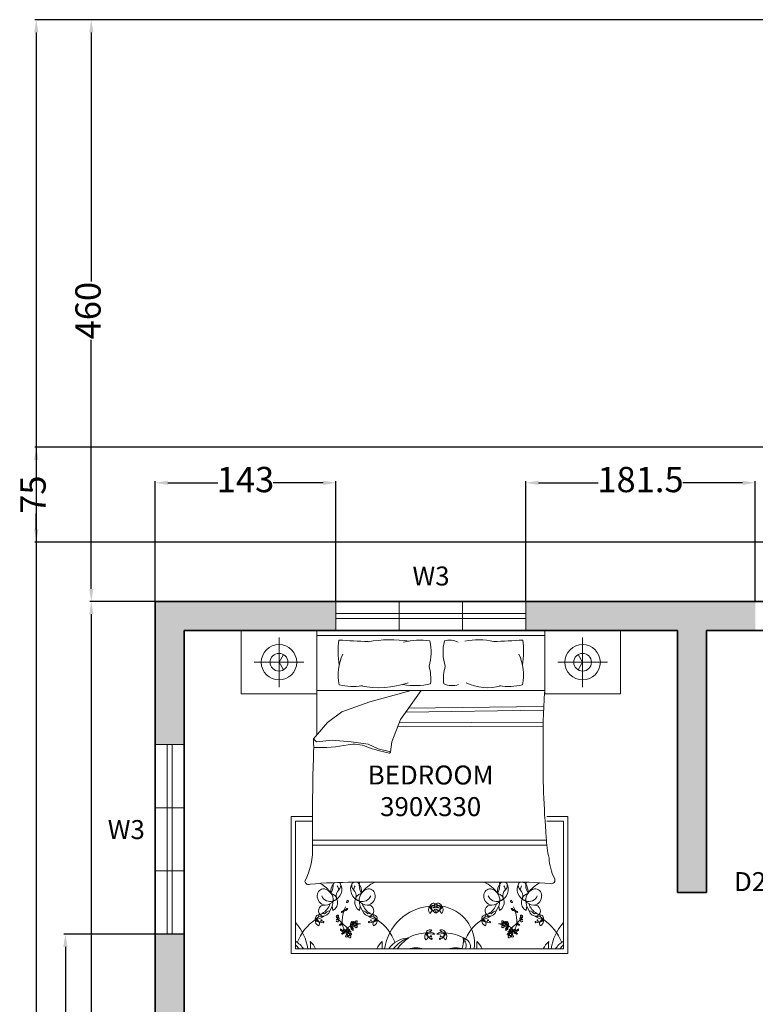
# Model space of a CAD drawing. Units: centimetres. Extents: x 2137 to 3697, y 183 to 2094.
# Tile 7 of 8: x 2163 to 2745, y 1208 to 1987. Entities that reach past the tile are written whole.
import ezdxf

# ---------------------------------------------------------------- set-up
doc = ezdxf.new("R2010")
doc.units = ezdxf.units.CM
for name, color, linetype, lineweight in [('A-ANNO-DIMS', 2, 'Continuous', 18), ('A-ANNO-TEXT', 7, 'Continuous', 18), ('A-AREA-IDEN', 7, 'Continuous', 25), ('A-FURN', 8, 'Continuous', 18), ('A-GLAZ', 4, 'Continuous', 18), ('A-WALL', 7, 'Continuous', 35), ('A-WALL-PATT', 52, 'Continuous', 13)]:
    doc.layers.add(name, color=color, linetype=linetype, lineweight=lineweight)
doc.styles.get("Standard").update_dxf_attribs({"font": 'arial.ttf'})
doc.dimstyles.new('ISO-25', dxfattribs={"dimtxt": 20, "dimasz": 10, "dimexe": 1.25, "dimexo": 0.625, "dimtad": 0, "dimtxsty": 'Standard', "dimcen": 2.5, "dimadec": 0, "dimazin": 0, "dimtfac": 1, "dimtmove": 0, "dimatfit": 3, "dimfxl": 1, "dimarcsym": 0})

# ---------------------------------------------------------------- blocks, each defined once
blk = doc.blocks.new('*D6')
at = {"layer": 'A-ANNO-DIMS', "color": 0, "lineweight": -2, "transparency": 16777216}
for p, q in [((2857.4, 1986.58), (2218.37, 1986.58)), ((2219.62, 1976.58), (2219.62, 1779.67)), ((2219.62, 1536.58), (2219.62, 1733.49)), ((2857.4, 1526.58), (2218.37, 1526.58))]:
    blk.add_line(p, q, dxfattribs=at)
at = {"layer": 'A-ANNO-DIMS', "color": 0, "transparency": 16777216}
for points in [[(2217.95, 1976.58), (2221.28, 1976.58), (2219.62, 1986.58)], [(2217.95, 1536.58), (2221.28, 1536.58), (2219.62, 1526.58)]]:
    blk.add_solid(points, dxfattribs=at)
at = {"layer": 'Defpoints', "color": 0, "transparency": 16777216}
for p in [(2858.02, 1986.58), (2219.62, 1526.58), (2858.02, 1526.58)]:
    blk.add_point(p, dxfattribs=at)
at = {"layer": 'A-ANNO-DIMS', "color": 0, "transparency": 16777216, "insert": (2219.62, 1756.58), "char_height": 20, "attachment_point": 5, "rotation": 90}
blk.add_mtext('460', dxfattribs=at)
blk = doc.blocks.new('*D7')
at = {"layer": 'A-ANNO-DIMS', "color": 0, "lineweight": -2, "transparency": 16777216}
for p, q in [((2269.4, 1526.58), (2218.41, 1526.58)), ((2219.66, 1516.58), (2219.66, 941.09)), ((2219.66, 306.58), (2219.66, 882.07)), ((2269.4, 296.58), (2218.41, 296.58))]:
    blk.add_line(p, q, dxfattribs=at)
at = {"layer": 'A-ANNO-DIMS', "color": 0, "transparency": 16777216}
for points in [[(2217.99, 1516.58), (2221.33, 1516.58), (2219.66, 1526.58)], [(2217.99, 306.58), (2221.33, 306.58), (2219.66, 296.58)]]:
    blk.add_solid(points, dxfattribs=at)
at = {"layer": 'Defpoints', "color": 0, "transparency": 16777216}
for p in [(2270.02, 1526.58), (2219.66, 296.58), (2270.02, 296.58)]:
    blk.add_point(p, dxfattribs=at)
at = {"layer": 'A-ANNO-DIMS', "color": 0, "transparency": 16777216, "insert": (2219.66, 911.58), "char_height": 20, "attachment_point": 5, "rotation": 90}
blk.add_mtext('1230', dxfattribs=at)
blk = doc.blocks.new('BED')
for p, q in [((2442.52, 2474.71), (2742.52, 2474.71)), ((2472.52, 2430.11), (2472.52, 2469.31)), ((2502.52, 2474.71), (2502.52, 2392.37)), ((2682.52, 2470.86), (2502.52, 2470.86)), ((2712.52, 2430.11), (2712.52, 2469.31)), ((2492.12, 2449.71), (2452.92, 2449.71)), ((2692.92, 2449.71), (2732.12, 2449.71)), ((2502.52, 2427.3), (2682.52, 2427.3)), ((2544.19, 2418.38), (2576.9, 2427.3)), ((2584.93, 2427.3), (2568.49, 2404.42)), ((2522.31, 2410.49), (2544.19, 2418.38)), ((2681.71, 2414.84), (2574.9, 2413.34)), ((2510.77, 2401.99), (2522.31, 2410.49)), ((2681.6, 2411.76), (2572.66, 2410.22)), ((2499.83, 2389.24), (2510.77, 2401.99)), ((2568.49, 2404.42), (2561.81, 2386.81)), ((2681.46, 2399.23), (2566.35, 2398.76)), ((2681.44, 2402.31), (2567.52, 2401.86)), ((2502.26, 2386.81), (2499.83, 2389.24)), ((2514.41, 2388.02), (2502.26, 2386.81)), ((2529.61, 2386.81), (2514.41, 2388.02)), ((2542.97, 2384.99), (2529.61, 2386.81)), ((2550.87, 2381.34), (2542.97, 2384.99)), ((2561.81, 2386.81), (2560.59, 2378.91)), ((2560.59, 2378.91), (2550.87, 2381.34)), ((2482.11, 2327.65), (2499.08, 2327.65)), ((2482.11, 2219.58), (2482.11, 2327.65)), ((2684.19, 2327.65), (2700.83, 2327.65)), ((2700.83, 2327.65), (2700.83, 2219.58)), ((2499.08, 2324.17), (2485.59, 2324.17)), ((2485.59, 2324.17), (2485.59, 2223.06)), ((2697.35, 2324.17), (2684.13, 2324.17)), ((2697.35, 2223.06), (2697.35, 2324.17)), ((2683.88, 2308.94), (2499.06, 2308.94)), ((2684.17, 2305.2), (2499.06, 2305.2)), ((2653.42, 2275.73), (2531.62, 2275.73)), ((2515.15, 2253.47), (2514.49, 2256.86)), ((2536.12, 2253.47), (2536.78, 2256.86)), ((2646.82, 2253.47), (2646.16, 2256.86)), ((2667.79, 2253.47), (2668.45, 2256.86)), ((2700.83, 2219.58), (2482.11, 2219.58)), ((2485.59, 2223.06), (2697.35, 2223.06))]:
    blk.add_line(p, q)
for points in [[(2502.52, 2424.71), (2442.52, 2424.71), (2442.52, 2474.71)], [(2682.52, 2474.71), (2682.52, 2424.71), (2742.52, 2424.71), (2742.52, 2474.71)], [(2472.52, 2449.71), (2476.02, 2455.77)], [(2712.52, 2449.71), (2709.02, 2455.77)], [(2472.52, 2449.71), (2476.02, 2443.65)], [(2712.52, 2449.71), (2709.02, 2443.65)]]:
    blk.add_lwpolyline(points)
for points in [[(2519.75, 2467.23, 0.074897), (2520.11, 2447.64, -0.472817)], [(2591.11, 2446.54, 0.14099), (2591.71, 2466.53, 0.235245)], [(2603.92, 2446.54, -0.14099), (2603.32, 2466.53, -0.235245)], [(2665.29, 2467.23, -0.074897), (2664.92, 2447.64, 0.472817)], [(2499.2, 2361.77, 0.001242), (2499.06, 2304.85, -0.127202), (2493.05, 2276.48)], [(2683.8, 2311.3, 0.056112), (2685.97, 2294.79, 0.095341), (2690.19, 2278.9)]]:
    blk.add_lwpolyline(points, format="xyb")
for centre, radius in [((2472.52, 2449.71), 14), ((2712.52, 2449.71), 14), ((2472.52, 2449.71), 7), ((2712.52, 2449.71), 7), ((2532.49, 2242.6), 0.764), ((2650.46, 2242.6), 0.764), ((2527.49, 2234.55), 0.764), ((2655.45, 2234.55), 0.764)]:
    blk.add_circle(centre, radius)
for centre, radius, start, end in [((2685.11, 5322.24), 2859.79, 266.68521, 267.14978), ((2560.85, 2358.67), 108.8, 82.21958, 99.49698), ((2583.83, 2413.66), 53.46, 81.52493, 103.95996), ((2607.44, 2452.27), 14.84, 63.34374, 106.10256), ((2629.68, 2414.74), 52.74, 76.34271, 101.1841), ((2499.93, 5322.24), 2859.79, 272.85022, 273.31479), ((2557.97, 2439.77), 38.67, 155.1316, 191.75834), ((2627.07, 2439.77), 38.67, 348.24166, 24.8684), ((2555.75, 2436.51), 36.76, 354.01289, 15.82928), ((2639.29, 2436.51), 36.76, 164.17072, 185.98711), ((2530.45, 2470.74), 40.2, 255.10393, 281.03689), ((2551.61, 2499.32), 69.73, 258.03974, 289.26152), ((2579.84, 2484.1), 52.9, 259.86169, 283.62376), ((2609.45, 2447.1), 15.9, 245.01826, 288.54073), ((2637.23, 2467.78), 38.19, 243.87611, 286.17464), ((2654.58, 2470.74), 40.2, 258.96311, 284.89607), ((3220.32, 2390.64), 539.05, 176.09997, 180.92818), ((2224.76, 2381.78), 275.17, 355.82941, 1.55305), ((2504.97, 2495.47), 113.22, 267.45188, 281.3392), ((2532.03, 2360.52), 24.42, 66.26158, 101.3392), ((2581.42, 2492.28), 116.34, 250.11942, 259.33829), ((2559.91, 2378.67), 0.724, 268.86235, 19.75363), ((3384.42, 2371.04), 703.17, 179.11454, 184.87351), ((2495.81, 2276.67), 2.77, 183.97998, 297.34124), ((2528.04, 1963.45), 312.3, 89.34325, 95.68869), ((2494.64, 2254.6), 22.71, 33.66712, 63.29966), ((2525.07, 2268.11), 11.57, 145.78505, 184.73037), ((2502.97, 2273.51), 12.43, 328.82178, 9.15542), ((2518.36, 2272.41), 3.61, 120.0293, 142.32497), ((2512.59, 2270.28), 9.56, 289.28218, 29.1751), ((2516.83, 2273.13), 4.49, 311.56531, 23.83541), ((2518.36, 2272.41), 3.61, 44.45169, 63.55801), ((2538.68, 2270.28), 9.56, 150.8249, 250.71782), ((2534.44, 2273.13), 4.49, 156.16459, 228.43469), ((2532.91, 2272.41), 3.61, 113.22901, 135.54831), ((2532.91, 2272.41), 3.61, 37.67503, 66.71436), ((2526.21, 2268.11), 11.57, 355.26963, 34.21495), ((2548.31, 2273.51), 12.43, 169.71335, 211.17822), ((2556.64, 2254.6), 22.71, 111.49413, 146.33288), ((2626.3, 2254.6), 22.71, 33.66712, 68.50587), ((2656.73, 2268.11), 11.57, 145.78505, 184.73037), ((2634.63, 2273.51), 12.43, 328.82178, 10.28665), ((2650.03, 2272.41), 3.61, 113.28564, 142.32497), ((2644.26, 2270.28), 9.56, 289.28218, 29.1751), ((2650.03, 2272.41), 3.61, 44.45169, 66.71436), ((2648.5, 2273.13), 4.49, 311.56531, 23.83541), ((2662.61, 1983.95), 291.92, 85.24024, 91.80351), ((2670.35, 2270.28), 9.56, 150.8249, 250.71782), ((2666.11, 2273.13), 4.49, 156.16459, 228.43469), ((2664.58, 2272.41), 3.61, 106.63434, 135.54831), ((2664.58, 2272.41), 3.61, 37.67503, 72.58143), ((2657.87, 2268.11), 11.57, 355.26963, 34.21495), ((2679.98, 2273.51), 12.43, 169.24899, 211.17822), ((2688.3, 2254.6), 22.71, 113.64533, 146.33288), ((2687.92, 2277.37), 2.73, 246.52186, 33.82642), ((2509.94, 2264.78), 7.17, 174.94485, 262.88575), ((2507.86, 2265.5), 5.07, 84.48557, 181.05378), ((2506.31, 2261.76), 9.02, 355.29334, 76.921), ((2511.44, 2259.94), 7.46, 299.90854, 73.1337), ((2523.89, 2265.16), 6.15, 131.56531, 195.14713), ((2511.15, 2268.55), 8.62, 7.43599, 29.91487), ((2527.38, 2265.16), 6.15, 344.85287, 48.43469), ((2540.13, 2268.55), 8.62, 150.08513, 172.56401), ((2539.84, 2259.94), 7.46, 106.8663, 240.09146), ((2544.97, 2261.76), 9.02, 103.079, 184.70666), ((2541.33, 2264.78), 7.17, 277.11425, 5.05515), ((2543.41, 2265.5), 5.07, 358.94622, 95.51443), ((2641.61, 2264.78), 7.17, 174.94485, 262.88575), ((2639.53, 2265.5), 5.07, 84.48557, 181.05378), ((2637.98, 2261.76), 9.02, 355.29334, 76.921), ((2643.1, 2259.94), 7.46, 299.90854, 73.1337), ((2655.56, 2265.16), 6.15, 131.56531, 195.14713), ((2642.81, 2268.55), 8.62, 7.43599, 29.91487), ((2659.05, 2265.16), 6.15, 344.85287, 48.43469), ((2671.79, 2268.55), 8.62, 150.08513, 172.56401), ((2671.51, 2259.94), 7.46, 106.8663, 240.09146), ((2676.63, 2261.76), 9.02, 103.079, 184.70666), ((2673, 2264.78), 7.17, 277.11425, 5.05515), ((2675.08, 2265.5), 5.07, 358.94622, 95.51443), ((2508.29, 2253.23), 4.5, 80.26398, 250.86884), ((2512.76, 2267.5), 6.96, 201.58187, 291.42215), ((2499.37, 2263.14), 14.16, 301.26137, 341.7045), ((2508.7, 2266.37), 8.71, 272.3591, 324.04014), ((2499.23, 2262), 16.1, 326.28828, 356.5076), ((2525.07, 2268.11), 11.57, 212.70113, 216.34448), ((2516.16, 2263.07), 1.86, 257.30406, 15.14713), ((2526.5, 2260.25), 0.578, 102.70507, 280.43845), ((2526.43, 2260.6), 0.94, 280.43845, 100.41356), ((2535.12, 2263.07), 1.86, 164.85287, 282.69594), ((2526.21, 2268.11), 11.57, 323.65552, 327.29887), ((2542.58, 2266.37), 8.71, 215.95986, 267.6409), ((2538.52, 2267.5), 6.96, 248.57785, 338.41813), ((2552.04, 2262), 16.1, 183.4924, 213.71172), ((2551.91, 2263.14), 14.16, 198.2955, 238.73863), ((2542.98, 2253.23), 4.5, 289.13116, 99.73602), ((2594.92, 2255.93), 3.25, 63.02737, 163.80375), ((2591.63, 2263.52), 6.69, 271.45846, 315.37266), ((2598.02, 2255.93), 3.25, 16.19625, 116.97263), ((2601.31, 2263.52), 6.69, 224.62734, 268.54154), ((2639.96, 2253.23), 4.5, 80.26398, 250.86884), ((2644.43, 2267.5), 6.96, 201.58187, 291.42215), ((2631.03, 2263.14), 14.16, 301.26137, 341.7045), ((2640.36, 2266.37), 8.71, 272.3591, 324.04014), ((2630.9, 2262), 16.1, 326.28828, 356.5076), ((2656.73, 2268.11), 11.57, 212.70113, 216.34448), ((2647.82, 2263.07), 1.86, 257.30406, 15.14713), ((2656.51, 2260.6), 0.94, 79.58644, 259.56155), ((2656.44, 2260.25), 0.578, 259.56155, 77.29493), ((2666.78, 2263.07), 1.86, 164.85287, 282.69594), ((2657.87, 2268.11), 11.57, 323.65552, 327.29887), ((2674.25, 2266.37), 8.71, 215.95986, 267.6409), ((2670.18, 2267.5), 6.96, 248.57785, 338.41813), ((2683.71, 2262), 16.1, 183.4924, 213.71172), ((2683.58, 2263.14), 14.16, 198.2955, 238.73863), ((2674.65, 2253.23), 4.5, 289.13116, 99.73602), ((2504.48, 2247), 3.25, 92.95159, 193.72796), ((2497.84, 2251.95), 6.69, 301.38267, 345.29688), ((2507.37, 2248.35), 2.76, 63.97555, 143.26805), ((2507.21, 2254.58), 5.62, 265.96902, 344.3045), ((2513.27, 2247.11), 5.99, 96.1662, 141.58255), ((2518.96, 2249.23), 0.59, 345.23556, 144.9248), ((2523.19, 2251.31), 1.58, 101.32561, 154.46214), ((2520.92, 2256.65), 4.74, 280.25878, 300.65599), ((2522.01, 2260.45), 8.46, 268.32639, 277.13024), ((2547.29, 2245.15), 24.85, 163.58418, 183.82768), ((2519.89, 2256.64), 4.82, 308.21012, 316.30712), ((2522.85, 2253.47), 1.44, 278.34322, 4.28685), ((2522.06, 2254.74), 2.51, 300.65599, 332.63414), ((2523.94, 2253.08), 0.611, 55.76575, 157.44165), ((2547.29, 2245.15), 24.85, 153.0032, 159.89408), ((2524.9, 2253.65), 0.611, 84.37838, 186.05427), ((2524.32, 2256.1), 2.51, 269.18588, 301.16403), ((2525.06, 2254.8), 1.44, 237.53317, 323.47681), ((2523.67, 2258.9), 4.82, 285.51291, 293.60991), ((2526.81, 2253.48), 1.58, 87.35788, 140.49441), ((2523.17, 2258), 4.74, 301.16403, 321.56124), ((2519.31, 2258.83), 8.46, 324.68979, 333.49364), ((2538.01, 2247.11), 5.99, 38.41745, 83.8338), ((2544.06, 2254.58), 5.62, 195.6955, 274.03098), ((2543.91, 2248.35), 2.76, 36.73195, 116.02445), ((2546.8, 2247), 3.25, 346.27204, 87.04841), ((2553.44, 2251.95), 6.69, 194.70312, 238.61733), ((2594.85, 2217.78), 39.18, 94.46233, 172.25504), ((2595.02, 2253.92), 4.34, 137.78732, 219.11446), ((2590.09, 2254.05), 3.27, 298.5391, 58.36268), ((2594.35, 2251.19), 6.19, 45.54113, 114.31008), ((2600, 2282.98), 27.41, 252.59304, 267.25817), ((2595, 2256.71), 3.2, 177.75849, 283.85198), ((2601.17, 2260.05), 9.91, 198.91595, 238.01098), ((2598.59, 2251.19), 6.19, 65.68992, 134.45887), ((2592.94, 2282.98), 27.41, 272.74183, 287.40696), ((2595.67, 2254.01), 0.424, 283.85198, 219.92454), ((2596.18, 2252.06), 0.487, 238.01098, 71.55918), ((2596.26, 2252.29), 0.236, 71.55918, 188.01668), ((2596.76, 2252.06), 0.487, 108.44082, 301.98902), ((2596.68, 2252.29), 0.236, 351.98332, 108.44082), ((2597.23, 2254.17), 0.255, 320.19092, 256.02088), ((2591.77, 2260.05), 9.91, 301.98902, 341.08405), ((2597.94, 2256.71), 3.2, 256.14802, 2.24151), ((2602.86, 2254.05), 3.27, 121.63732, 241.4609), ((2597.92, 2253.92), 4.34, 320.88554, 42.21268), ((2596.83, 2226.82), 30.32, 352.86355, 81.81966), ((2636.14, 2247), 3.25, 92.95159, 193.72796), ((2629.51, 2251.95), 6.69, 301.38267, 345.29688), ((2639.03, 2248.35), 2.76, 63.97555, 143.26805), ((2638.88, 2254.58), 5.62, 265.96902, 344.3045), ((2644.93, 2247.11), 5.99, 96.1662, 141.58255), ((2656.13, 2253.48), 1.58, 39.50559, 92.64212), ((2659.77, 2258), 4.74, 218.43876, 238.83597), ((2663.63, 2258.83), 8.46, 206.50636, 215.31021), ((2657.88, 2254.8), 1.44, 216.52319, 302.46683), ((2658.62, 2256.1), 2.51, 238.83597, 270.81412), ((2659.27, 2258.9), 4.82, 246.39009, 254.48709), ((2635.65, 2245.15), 24.85, 20.10592, 26.9968), ((2658.05, 2253.65), 0.611, 353.94573, 95.62162), ((2659, 2253.08), 0.611, 22.55835, 124.23425), ((2660.09, 2253.47), 1.44, 175.71315, 261.65678), ((2660.89, 2254.74), 2.51, 207.36586, 239.34401), ((2635.65, 2245.15), 24.85, 356.17232, 16.41582), ((2663.05, 2256.64), 4.82, 223.69288, 231.78988), ((2662.02, 2256.65), 4.74, 239.34401, 259.74122), ((2660.93, 2260.45), 8.46, 262.86976, 271.67361), ((2659.76, 2251.31), 1.58, 25.53786, 78.67439), ((2663.98, 2249.23), 0.59, 35.0752, 194.76444), ((2675.73, 2254.58), 5.62, 195.6955, 274.03098), ((2669.67, 2247.11), 5.99, 38.41745, 83.8338), ((2675.58, 2248.35), 2.76, 36.73195, 116.02445), ((2685.1, 2251.95), 6.69, 194.70312, 238.61733), ((2678.46, 2247), 3.25, 346.27204, 87.04841), ((2456.43, 2217.78), 39.18, 7.74496, 41.8856), ((2523.45, 2213.9), 39.18, 124.38655, 158.59079), ((2505.57, 2245.31), 4.34, 167.71153, 249.03868), ((2506.35, 2242.61), 6.19, 75.46535, 144.23429), ((2495.38, 2272.99), 27.41, 282.51726, 297.18239), ((2501.23, 2242.96), 3.27, 328.46331, 88.28689), ((2507.84, 2253.69), 9.91, 228.84017, 267.9352), ((2504.16, 2247.72), 3.2, 207.6827, 313.77619), ((2506.09, 2245.71), 0.424, 313.77619, 249.71835), ((2507.46, 2244.52), 0.236, 101.4834, 217.94089), ((2507.5, 2244.28), 0.487, 267.9352, 101.4834), ((2518.73, 2248.32), 1.27, 101.56373, 142.6358), ((2517.68, 2247.14), 0.764, 273.27684, 86.72316), ((2518.72, 2245.73), 1.26, 217.76209, 259.04026), ((2518.57, 2247.86), 0.73, 91.10805, 181.86747), ((2520.08, 2247.41), 2.32, 203.42757, 227.61037), ((2519.34, 2246.4), 1.58, 80.3487, 133.65382), ((2519.06, 2247.7), 1.25, 229.78892, 317.67915), ((2517.71, 2249.32), 1.84, 288.72627, 352.50315), ((2517.65, 2245.06), 1.78, 355.05304, 68.36176), ((2519.04, 2244.75), 2.5, 83.08516, 105.71709), ((2518.83, 2244.95), 0.586, 232.47371, 355.05304), ((2501.72, 2224.01), 28.48, 43.15413, 52.0459), ((2519.5, 2247.3), 0.658, 317.67915, 80.3487), ((2521.4, 2241.21), 1.58, 101.32561, 154.46214), ((2519.13, 2246.56), 4.74, 280.25878, 300.65599), ((2520.22, 2250.35), 8.46, 268.32639, 277.13024), ((2518.11, 2246.55), 4.82, 308.21012, 316.30712), ((2521.07, 2243.38), 1.44, 278.34322, 4.28685), ((2520.27, 2244.64), 2.51, 300.65599, 332.63414), ((2522.16, 2242.98), 0.611, 55.76575, 157.44165), ((2534.91, 2244.52), 12.46, 184.75602, 209.20408), ((2552.85, 2271.04), 40.99, 222.24124, 232.17444), ((2528.5, 2242.96), 2.12, 272.84988, 356.12261), ((2526.64, 2243.74), 3.48, 304.53686, 16.36991), ((2527, 2242.14), 2.05, 321.76073, 7.92519), ((2531.47, 2242.76), 2.46, 127.31045, 187.92519), ((2528.09, 2243.04), 2.53, 355.01064, 41.65801), ((2532.28, 2240.29), 2.41, 104.75581, 148.0499), ((2531.64, 2243.66), 1.04, 126.10456, 271.42811), ((2531.53, 2243.95), 0.749, 353.75256, 131.70535), ((2531.35, 2241.96), 0.506, 262.90601, 7.13198), ((2530.82, 2243.06), 1.05, 0.06451, 61.15075), ((2531.07, 2243.95), 1.2, 311.84125, 355.78771), ((2533.54, 2243.78), 1.27, 101.56373, 176.36503), ((2533.38, 2243.32), 0.73, 91.10805, 181.86747), ((2534.89, 2242.87), 2.32, 203.42757, 227.61037), ((2534.15, 2241.86), 1.58, 80.3487, 133.65382), ((2533.87, 2243.16), 1.25, 229.78892, 317.67915), ((2532.52, 2244.78), 1.84, 288.72627, 352.50315), ((2532.46, 2240.51), 1.78, 355.05304, 68.36176), ((2533.85, 2240.21), 2.5, 83.08516, 105.71709), ((2533.77, 2244.69), 0.59, 345.23556, 144.9248), ((2534.31, 2242.76), 0.658, 317.67915, 80.3487), ((2536.2, 2227.98), 14.94, 87.10709, 94.75853), ((2543.77, 2244.28), 0.487, 78.5166, 272.0648), ((2544.93, 2242.61), 6.19, 35.76571, 104.53465), ((2555.89, 2272.99), 27.41, 242.81761, 257.48274), ((2543.43, 2253.69), 9.91, 272.0648, 311.15983), ((2543.82, 2244.52), 0.236, 322.05911, 78.5166), ((2547.11, 2247.72), 3.2, 226.22381, 332.3173), ((2545.24, 2245.88), 0.255, 290.26671, 226.22708), ((2550.05, 2242.96), 3.27, 91.71311, 211.53669), ((2545.71, 2245.31), 4.34, 290.96132, 12.28847), ((2527.83, 2213.9), 39.18, 21.40921, 55.61345), ((2655.12, 2213.9), 39.18, 124.38655, 158.59079), ((2637.23, 2245.31), 4.34, 167.71153, 249.03868), ((2638.02, 2242.61), 6.19, 75.46535, 144.23429), ((2627.05, 2272.99), 27.41, 282.51726, 297.18239), ((2635.83, 2247.72), 3.2, 207.6827, 313.77619), ((2639.51, 2253.69), 9.91, 228.84017, 267.9352), ((2632.89, 2242.96), 3.27, 328.46331, 88.28689), ((2637.75, 2245.71), 0.424, 313.77619, 249.71835), ((2639.12, 2244.52), 0.236, 101.4834, 217.94089), ((2639.17, 2244.28), 0.487, 267.9352, 101.4834), ((2646.75, 2227.98), 14.94, 85.24147, 92.89291), ((2648.64, 2242.76), 0.658, 99.6513, 222.32085), ((2649.07, 2243.16), 1.25, 222.32085, 310.21108), ((2648.79, 2241.86), 1.58, 46.34618, 99.6513), ((2649.17, 2244.69), 0.59, 35.0752, 194.76444), ((2650.42, 2244.78), 1.84, 187.49685, 251.27373), ((2650.48, 2240.51), 1.78, 111.63824, 184.94696), ((2649.09, 2240.21), 2.5, 74.28291, 96.91484), ((2649.56, 2243.32), 0.73, 358.13253, 88.89195), ((2648.05, 2242.87), 2.32, 312.38963, 336.57243), ((2649.4, 2243.78), 1.27, 3.63497, 78.43627), ((2651.41, 2243.95), 0.749, 48.29465, 186.24744), ((2651.87, 2243.95), 1.2, 184.21229, 228.15875), ((2652.12, 2243.06), 1.05, 118.84925, 179.93549), ((2651.59, 2241.96), 0.506, 172.86802, 277.09399), ((2651.3, 2243.66), 1.04, 268.57189, 53.89544), ((2650.66, 2240.29), 2.41, 31.9501, 75.24419), ((2654.85, 2243.04), 2.53, 138.34199, 184.98936), ((2654.44, 2242.96), 2.12, 183.87739, 267.15012), ((2656.3, 2243.74), 3.48, 163.63009, 235.46314), ((2651.47, 2242.76), 2.46, 352.07481, 52.68955), ((2655.94, 2242.14), 2.05, 172.07481, 218.23927), ((2630.09, 2271.04), 40.99, 307.82556, 317.75876), ((2648.03, 2244.52), 12.46, 330.79592, 355.24398), ((2681.22, 2224.01), 28.48, 127.9541, 136.84587), ((2660.78, 2242.98), 0.611, 22.55835, 124.23425), ((2661.88, 2243.38), 1.44, 175.71315, 261.65678), ((2662.67, 2244.64), 2.51, 207.36586, 239.34401), ((2664.83, 2246.55), 4.82, 223.69288, 231.78988), ((2663.81, 2246.56), 4.74, 239.34401, 259.74122), ((2662.72, 2250.35), 8.46, 262.86976, 271.67361), ((2661.54, 2241.21), 1.58, 25.53786, 78.67439), ((2663.45, 2247.3), 0.658, 99.6513, 222.32085), ((2663.88, 2247.7), 1.25, 222.32085, 310.21108), ((2663.6, 2246.4), 1.58, 46.34618, 99.6513), ((2665.23, 2249.32), 1.84, 187.49685, 251.27373), ((2665.29, 2245.06), 1.78, 111.63824, 184.94696), ((2664.11, 2244.95), 0.586, 184.94696, 307.52629), ((2663.9, 2244.75), 2.5, 74.28291, 96.91484), ((2664.38, 2247.86), 0.73, 358.13253, 88.89195), ((2662.86, 2247.41), 2.32, 312.38963, 336.57243), ((2664.21, 2248.32), 1.27, 37.3642, 78.43627), ((2664.23, 2245.73), 1.26, 280.95974, 322.23791), ((2665.27, 2247.14), 0.764, 93.27684, 266.72316), ((2675.44, 2244.28), 0.487, 78.5166, 272.0648), ((2676.59, 2242.61), 6.19, 35.76571, 104.53465), ((2687.56, 2272.99), 27.41, 242.81761, 257.48274), ((2675.1, 2253.69), 9.91, 272.0648, 311.15983), ((2675.49, 2244.52), 0.236, 322.05911, 78.5166), ((2678.78, 2247.72), 3.2, 226.22381, 332.3173), ((2676.9, 2245.88), 0.255, 290.26671, 226.22708), ((2681.72, 2242.96), 3.27, 91.71311, 211.53669), ((2677.37, 2245.31), 4.34, 290.96132, 12.28847), ((2659.49, 2213.9), 39.18, 21.40921, 55.61345), ((2726.52, 2217.78), 39.18, 138.1144, 172.25504), ((2521.93, 2238.45), 0.853, 146.86359, 236.90213), ((2533.96, 2257.24), 22.32, 235.1882, 238.88441), ((2523.39, 2239.69), 2.31, 199.47987, 267.68284), ((2523.14, 2238.82), 1.99, 212.81548, 277.39917), ((2521.98, 2237.49), 2.31, 266.97007, 338.29129), ((2509.81, 2253.97), 22.32, 302.6784, 306.37461), ((2522.56, 2235.66), 0.853, 214.3538, 304.39233), ((2522.88, 2238.89), 0.883, 238.88441, 314.26458), ((2522.69, 2236.91), 1.99, 280.30568, 17.1958), ((2522.52, 2236.71), 0.883, 306.37461, 21.75478), ((2523.96, 2237.28), 0.666, 19.36054, 201.75478), ((2523.96, 2237.78), 0.666, 311.87034, 134.26458), ((2536.49, 2231.71), 13.31, 153.78194, 158.29129), ((2525.9, 2240.8), 3.48, 247.23048, 319.06353), ((2524.75, 2239.63), 2.05, 264.45436, 310.61881), ((2534.91, 2244.52), 12.46, 214.00334, 222.49171), ((2526.25, 2238.81), 2.12, 218.32082, 298.81623), ((2536.2, 2227.98), 14.94, 120.54402, 139.81798), ((2527.28, 2232.24), 2.41, 104.75581, 148.0499), ((2526.65, 2235.61), 1.04, 126.10456, 271.42811), ((2526.53, 2235.89), 0.749, 353.75256, 131.70535), ((2527.69, 2236.2), 2.46, 70.00407, 130.61881), ((2525.83, 2235), 1.05, 0.06451, 61.15075), ((2526.08, 2235.9), 1.2, 311.84125, 355.78771), ((2526.09, 2239.2), 2.53, 297.70426, 344.35163), ((2528.55, 2235.73), 1.27, 101.56373, 176.36503), ((2528.38, 2235.27), 0.73, 91.10805, 181.86747), ((2529.15, 2233.8), 1.58, 80.3487, 133.65382), ((2528.87, 2235.11), 1.25, 229.78892, 317.67915), ((2527.52, 2236.73), 1.84, 288.72627, 352.50315), ((2527.46, 2232.46), 1.78, 355.05304, 68.36176), ((2528.85, 2232.16), 2.5, 83.08516, 105.71709), ((2528.77, 2236.64), 0.59, 345.23556, 144.9248), ((2527.43, 2239.19), 2.05, 8.72271, 54.88717), ((2527.54, 2237.55), 3.48, 0.278, 72.11105), ((2529.1, 2238.83), 2.12, 20.5253, 88.5375), ((2529.31, 2234.71), 0.658, 317.67915, 80.3487), ((2531.89, 2239.88), 2.46, 188.72271, 249.33746), ((2530.88, 2241.17), 0.757, 148.0499, 225.62681), ((2536.2, 2227.98), 14.94, 113.05007, 113.84774), ((2530.93, 2242.02), 1.51, 247.40857, 351.43859), ((2528.73, 2238.64), 2.53, 334.9899, 21.63727), ((2533.53, 2241.19), 1.26, 151.21959, 259.04026), ((2533.64, 2240.41), 0.586, 232.47371, 355.05304), ((2591.85, 2196.79), 39.18, 94.46233, 117.4146), ((2592.02, 2232.93), 4.34, 137.78732, 219.11446), ((2587.09, 2233.07), 3.27, 298.5391, 58.36268), ((2591.92, 2234.94), 3.25, 63.02737, 163.80375), ((2588.63, 2242.54), 6.69, 271.45846, 315.37266), ((2591.35, 2230.21), 6.19, 45.54113, 114.31008), ((2598.17, 2239.06), 9.91, 198.91595, 238.01098), ((2597, 2262), 27.41, 252.59304, 267.25817), ((2592, 2235.73), 3.2, 177.75849, 283.85198), ((2601.59, 2230.21), 6.19, 65.68992, 134.45887), ((2595.94, 2262), 27.41, 272.74183, 287.40696), ((2601.02, 2234.94), 3.25, 16.19625, 116.97263), ((2604.31, 2242.54), 6.69, 224.62734, 268.54154), ((2594.77, 2239.06), 9.91, 301.98902, 341.08405), ((2600.94, 2235.73), 3.2, 256.14802, 2.24151), ((2605.86, 2233.07), 3.27, 121.63732, 241.4609), ((2600.92, 2232.93), 4.34, 320.88554, 42.21268), ((2601.09, 2196.79), 39.18, 62.5854, 85.53767), ((2649.3, 2240.41), 0.586, 184.94696, 307.52629), ((2649.41, 2241.19), 1.26, 280.95974, 28.78041), ((2652.01, 2242.02), 1.51, 188.56141, 292.59143), ((2654.21, 2238.64), 2.53, 158.36273, 205.0101), ((2653.84, 2238.83), 2.12, 91.4625, 159.4747), ((2655.4, 2237.55), 3.48, 107.88895, 179.722), ((2651.05, 2239.88), 2.46, 290.66254, 351.27729), ((2652.06, 2241.17), 0.757, 314.37319, 31.9501), ((2646.75, 2227.98), 14.94, 66.15226, 66.94993), ((2653.63, 2234.71), 0.658, 99.6513, 222.32085), ((2654.07, 2235.11), 1.25, 222.32085, 310.21108), ((2655.51, 2239.19), 2.05, 125.11283, 171.27729), ((2653.79, 2233.8), 1.58, 46.34618, 99.6513), ((2654.17, 2236.64), 0.59, 35.0752, 194.76444), ((2655.42, 2236.73), 1.84, 187.49685, 251.27373), ((2655.48, 2232.46), 1.78, 111.63824, 184.94696), ((2654.09, 2232.16), 2.5, 74.28291, 96.91484), ((2646.75, 2227.98), 14.94, 40.18202, 59.45598), ((2655.26, 2236.2), 2.46, 49.38119, 109.99593), ((2657.04, 2240.8), 3.48, 220.93647, 292.76952), ((2656.85, 2239.2), 2.53, 195.64837, 242.29574), ((2654.56, 2235.27), 0.73, 358.13253, 88.89195), ((2654.4, 2235.73), 1.27, 3.63497, 78.43627), ((2656.41, 2235.89), 0.749, 48.29465, 186.24744), ((2656.69, 2238.81), 2.12, 241.18377, 321.67918), ((2656.87, 2235.9), 1.2, 184.21229, 228.15875), ((2657.12, 2235), 1.05, 118.84925, 179.93549), ((2656.3, 2235.61), 1.04, 268.57189, 53.89544), ((2655.66, 2232.24), 2.41, 31.9501, 75.24419), ((2658.19, 2239.63), 2.05, 229.38119, 275.54564), ((2648.03, 2244.52), 12.46, 317.50829, 325.99666), ((2660.25, 2236.91), 1.99, 162.8042, 259.69432), ((2658.98, 2237.78), 0.666, 45.73542, 228.12966), ((2658.98, 2237.28), 0.666, 338.24522, 160.63946), ((2646.45, 2231.71), 13.31, 21.70871, 26.21806), ((2660.96, 2237.49), 2.31, 201.70871, 273.02993), ((2660.06, 2238.89), 0.883, 225.73542, 301.11559), ((2660.42, 2236.71), 0.883, 158.24522, 233.62539), ((2659.81, 2238.82), 1.99, 262.60083, 327.18452), ((2659.55, 2239.69), 2.31, 272.31716, 340.52013), ((2673.14, 2253.97), 22.32, 233.62539, 237.3216), ((2660.38, 2235.66), 0.853, 235.60767, 325.6462), ((2648.98, 2257.24), 22.32, 301.11559, 304.8118), ((2661.01, 2238.45), 0.853, 303.09787, 33.13641), ((2476.08, 2212.53), 19.09, 33.46172, 60.11157), ((2486.77, 2216.95), 15.93, 22.55474, 48.95456), ((2443.14, 2225.51), 54.2, 357.40811, 3.65191), ((2525.88, 2233.11), 0.757, 148.0499, 225.62681), ((2525.93, 2233.96), 1.51, 247.40857, 351.43859), ((2526.36, 2233.9), 0.506, 262.90601, 7.13198), ((2528.53, 2233.13), 1.26, 151.21959, 259.04026), ((2529.89, 2234.81), 2.32, 203.42757, 227.61037), ((2528.65, 2232.36), 0.586, 232.47371, 355.05304), ((2564.51, 2216.95), 15.93, 131.04544, 157.44526), ((2608.14, 2225.51), 54.2, 176.34809, 182.59189), ((2575.2, 2212.53), 19.09, 91.27197, 146.53828), ((2582.06, 2208.97), 23.79, 107.85038, 143.69643), ((2594.57, 2202.28), 35.39, 124.01234, 144.05304), ((2592.67, 2233.03), 0.424, 283.85198, 219.92454), ((2593.18, 2231.07), 0.487, 238.01098, 71.55918), ((2593.26, 2231.31), 0.236, 71.55918, 188.01668), ((2599.76, 2231.07), 0.487, 108.44082, 301.98902), ((2599.68, 2231.31), 0.236, 351.98332, 108.44082), ((2600.23, 2233.19), 0.255, 320.19092, 256.02088), ((2600.75, 2229.59), 17.54, 338.11703, 6.61954), ((2616.84, 2224.71), 7.03, 346.38982, 79.07385), ((2611.55, 2225.68), 8.89, 342.86088, 41.90487), ((2574.8, 2225.51), 54.2, 357.40811, 3.65191), ((2618.44, 2216.95), 15.93, 22.55474, 48.95456), ((2654.29, 2232.36), 0.586, 184.94696, 307.52629), ((2653.05, 2234.81), 2.32, 312.38963, 336.57243), ((2654.41, 2233.13), 1.26, 280.95974, 28.78041), ((2657.01, 2233.96), 1.51, 188.56141, 292.59143), ((2656.58, 2233.9), 0.506, 172.86802, 277.09399), ((2657.06, 2233.11), 0.757, 314.37319, 31.9501), ((2696.17, 2216.95), 15.93, 131.04544, 157.44526), ((2739.8, 2225.51), 54.2, 176.34809, 182.59189), ((2706.86, 2212.53), 19.09, 119.88843, 146.53828), ((2469.21, 2208.97), 23.79, 36.30357, 46.48142), ((2580.89, 2202.46), 21.54, 73.54311, 107.0202), ((2589.43, 2191.36), 31.85, 94.37872, 95.63574), ((2606.21, 2169.53), 56.92, 109.72171, 109.90284), ((2612.05, 2202.46), 21.54, 72.9798, 106.45689), ((2603.51, 2191.36), 31.85, 84.36426, 85.62128), ((2586.74, 2169.53), 56.92, 70.09716, 70.27829), ((2713.73, 2208.97), 23.79, 133.51858, 143.69643)]:
    blk.add_arc(centre, radius, start, end)
blk = doc.blocks.new('WIN-W3-150CM')
for p, q in [((0, 23), (0, 0)), ((50, 23), (50, 0)), ((100, 23), (100, 0)), ((150, 23), (150, 0)), ((0, 13.5), (150, 13.5)), ((0, 9.5), (150, 9.5))]:
    blk.add_line(p, q)
blk = doc.blocks.new('*D38')
at = {"layer": 'A-ANNO-DIMS', "color": 0, "lineweight": -2, "transparency": 16777216}
for p, q in [((2857.4, 1986.58), (2174.92, 1986.58)), ((2176.17, 1976.58), (2176.17, 1171.09)), ((2176.17, 306.58), (2176.17, 1112.07)), ((2269.4, 296.58), (2174.92, 296.58))]:
    blk.add_line(p, q, dxfattribs=at)
at = {"layer": 'A-ANNO-DIMS', "color": 0, "transparency": 16777216}
for points in [[(2174.51, 1976.58), (2177.84, 1976.58), (2176.17, 1986.58)], [(2174.51, 306.58), (2177.84, 306.58), (2176.17, 296.58)]]:
    blk.add_solid(points, dxfattribs=at)
at = {"layer": 'Defpoints', "color": 0, "transparency": 16777216}
for p in [(2176.17, 1986.58), (2858.02, 1986.58), (2270.02, 296.58)]:
    blk.add_point(p, dxfattribs=at)
at = {"layer": 'A-ANNO-DIMS', "color": 0, "transparency": 16777216, "insert": (2176.17, 1141.58), "char_height": 20, "attachment_point": 5, "rotation": 90}
blk.add_mtext('1690', dxfattribs=at)
blk = doc.blocks.new('*D41')
at = {"layer": 'A-ANNO-DIMS', "color": 0, "lineweight": -2, "transparency": 16777216}
for p, q in [((3371.4, 1648.58), (2174.92, 1648.58)), ((2176.17, 1638.58), (2176.17, 1626.02)), ((2176.17, 1583.58), (2176.17, 1596.14)), ((3371.4, 1573.58), (2174.92, 1573.58))]:
    blk.add_line(p, q, dxfattribs=at)
at = {"layer": 'A-ANNO-DIMS', "color": 0, "transparency": 16777216}
for points in [[(2174.51, 1638.58), (2177.84, 1638.58), (2176.17, 1648.58)], [(2174.51, 1583.58), (2177.84, 1583.58), (2176.17, 1573.58)]]:
    blk.add_solid(points, dxfattribs=at)
at = {"layer": 'Defpoints', "color": 0, "transparency": 16777216}
for p in [(2176.17, 1648.58), (3372.02, 1648.58), (3372.02, 1573.58)]:
    blk.add_point(p, dxfattribs=at)
at = {"layer": 'A-ANNO-DIMS', "color": 0, "transparency": 16777216, "insert": (2176.17, 1611.08), "char_height": 20, "attachment_point": 5, "rotation": 90}
blk.add_mtext('75', dxfattribs=at)
blk = doc.blocks.new('*D52')
at = {"layer": 'A-ANNO-DIMS', "color": 0, "lineweight": -2, "transparency": 16777216}
for p, q in [((2292.4, 1263.58), (2197.92, 1263.58)), ((2199.17, 1253.58), (2199.17, 1191.38)), ((2199.17, 1085.58), (2199.17, 1147.78)), ((2292.4, 1075.58), (2197.92, 1075.58))]:
    blk.add_line(p, q, dxfattribs=at)
at = {"layer": 'A-ANNO-DIMS', "color": 0, "transparency": 16777216}
for points in [[(2197.51, 1253.58), (2200.84, 1253.58), (2199.17, 1263.58)], [(2197.51, 1085.58), (2200.84, 1085.58), (2199.17, 1075.58)]]:
    blk.add_solid(points, dxfattribs=at)
at = {"layer": 'Defpoints', "color": 0, "transparency": 16777216}
for p in [(2199.17, 1263.58), (2293.02, 1263.58), (2293.02, 1075.58)]:
    blk.add_point(p, dxfattribs=at)
at = {"layer": 'A-ANNO-DIMS', "color": 0, "transparency": 16777216, "insert": (2199.17, 1169.58), "char_height": 20, "attachment_point": 5, "rotation": 90}
blk.add_mtext('188', dxfattribs=at)
blk = doc.blocks.new('*D55')
at = {"layer": 'A-ANNO-DIMS', "color": 0, "lineweight": -2, "transparency": 16777216}
for p, q in [((2270.02, 1527.2), (2270.02, 1621.68)), ((2280.02, 1620.43), (2319.74, 1620.43)), ((2403.02, 1620.43), (2363.3, 1620.43)), ((2413.02, 1527.2), (2413.02, 1621.68))]:
    blk.add_line(p, q, dxfattribs=at)
at = {"layer": 'A-ANNO-DIMS', "color": 0, "transparency": 16777216}
for points in [[(2280.02, 1622.1), (2280.02, 1618.76), (2270.02, 1620.43)], [(2403.02, 1622.1), (2403.02, 1618.76), (2413.02, 1620.43)]]:
    blk.add_solid(points, dxfattribs=at)
at = {"layer": 'Defpoints', "color": 0, "transparency": 16777216}
for p in [(2413.02, 1620.43), (2270.02, 1526.58), (2413.02, 1526.58)]:
    blk.add_point(p, dxfattribs=at)
at = {"layer": 'A-ANNO-DIMS', "color": 0, "transparency": 16777216, "insert": (2341.52, 1620.43), "char_height": 20, "attachment_point": 5}
blk.add_mtext('143', dxfattribs=at)
blk = doc.blocks.new('*D56')
at = {"layer": 'A-ANNO-DIMS', "color": 0, "lineweight": -2, "transparency": 16777216}
for p, q in [((2563.02, 1527.2), (2563.02, 1621.68)), ((2573.02, 1620.43), (2620.27, 1620.43)), ((2734.52, 1620.43), (2687.28, 1620.43)), ((2744.52, 1527.2), (2744.52, 1621.68))]:
    blk.add_line(p, q, dxfattribs=at)
at = {"layer": 'A-ANNO-DIMS', "color": 0, "transparency": 16777216}
for points in [[(2573.02, 1622.1), (2573.02, 1618.76), (2563.02, 1620.43)], [(2734.52, 1622.1), (2734.52, 1618.76), (2744.52, 1620.43)]]:
    blk.add_solid(points, dxfattribs=at)
at = {"layer": 'Defpoints', "color": 0, "transparency": 16777216}
for p in [(2744.52, 1620.43), (2563.02, 1526.58), (2744.52, 1526.58)]:
    blk.add_point(p, dxfattribs=at)
at = {"layer": 'A-ANNO-DIMS', "color": 0, "transparency": 16777216, "insert": (2653.77, 1620.43), "char_height": 20, "attachment_point": 5}
blk.add_mtext('181.5', dxfattribs=at)

msp = doc.modelspace()

# ---------------------------------------------------------------- hatches: boundary and pattern name
at = {"layer": 'A-WALL-PATT'}
h = msp.add_hatch(color=256, dxfattribs=at)
h.dxf.hatch_style = 1
h.paths.add_polyline_path([(2413.023, 1526.579), (2270.023, 1526.579), (2270.023, 1413.579), (2293.023, 1413.579), (2293.023, 1503.579), (2413.023, 1503.579)])
h.paths.add_polyline_path([(2744.523, 1526.579), (2563.023, 1526.579), (2563.023, 1503.579), (2638.023, 1503.579), (2683.023, 1503.579), (2683.023, 1296.579), (2706.023, 1296.579), (2706.023, 1503.579), (2744.523, 1503.579)])
h.paths.add_polyline_path([(2881.023, 1541.602), (2858.023, 1541.602), (2858.023, 1526.579), (2819.523, 1526.579), (2819.523, 1503.579), (2858.023, 1503.579), (2858.023, 1311.579), (2781.023, 1311.579), (2781.023, 1296.579), (2858.023, 1296.579), (2858.023, 1273.579), (2881.023, 1273.579)])
h.paths.add_polyline_path([(3207.023, 1745.579), (2881.023, 1745.579), (2881.023, 1963.579), (2913.523, 1963.579), (2913.523, 1986.579), (2858.023, 1986.579), (2858.023, 1691.602), (2881.023, 1691.602), (2881.023, 1722.579), (3184.023, 1722.579), (3184.023, 1321.579), (3207.023, 1321.579)])
h.paths.add_polyline_path([(3072.523, 1986.579), (2988.523, 1986.579), (2988.523, 1963.579), (3021.023, 1963.579), (3021.023, 1820.579), (3036.023, 1820.579), (3036.023, 1963.579), (3072.523, 1963.579)], flags=17)
h.paths.add_polyline_path([(3207.023, 1986.579), (3147.523, 1986.579), (3147.523, 1963.579), (3184.023, 1963.579), (3184.023, 1845.579), (3207.023, 1845.579)], flags=17)
h.paths.add_polyline_path([(3590.023, 1986.579), (3307.023, 1986.579), (3307.023, 1963.579), (3567.023, 1963.579), (3567.023, 1888.579), (3590.023, 1888.579), (3590.023, 1963.579)])
h.paths.add_polyline_path([(3590.023, 1738.579), (3567.023, 1738.579), (3567.023, 1663.579), (3372.023, 1663.579), (3372.023, 1648.579), (3567.023, 1648.579), (3567.023, 1514.579), (3387.023, 1514.579), (3387.023, 1573.579), (3372.023, 1573.579), (3372.023, 1514.579), (3307.023, 1514.579), (3307.023, 1491.579), (3567.023, 1491.579), (3567.023, 1431.579), (3590.023, 1431.579)])
h.paths.add_polyline_path([(3590.023, 1281.579), (3567.023, 1281.579), (3567.023, 1221.579), (3184.023, 1221.579), (3184.023, 922.579), (3207.023, 922.579), (3207.023, 1198.579), (3567.023, 1198.579), (3567.023, 1055.075), (3590.023, 1055.075)])
h.paths.add_polyline_path([(3590.023, 905.075), (3567.023, 905.075), (3567.023, 774.852), (3590.023, 774.852)])
h.paths.add_polyline_path([(3590.023, 624.852), (3567.023, 624.852), (3567.023, 599.579), (3184.023, 599.579), (3184.023, 576.579), (3590.023, 576.579)])
h.paths.add_polyline_path([(3590.023, 443.579), (3567.023, 443.579), (3567.023, 420.579), (3590.023, 420.579)])
h.paths.add_polyline_path([(3225.908, 443.579), (3202.908, 443.579), (3202.908, 420.579), (3225.908, 420.579)])
h.paths.add_polyline_path([(3039.023, 599.579), (3016.023, 599.579), (3016.023, 443.579), (2937.023, 443.579), (2937.023, 420.579), (3039.023, 420.579)])
h.paths.add_polyline_path([(2787.023, 443.579), (2708.023, 443.579), (2708.023, 850.579), (2685.023, 850.579), (2685.023, 319.579), (2564.023, 319.579), (2564.023, 296.579), (2708.023, 296.579), (2708.023, 420.579), (2787.023, 420.579)])
h.paths.add_polyline_path([(2414.023, 319.579), (2293.023, 319.579), (2293.023, 412.079), (2270.023, 412.079), (2270.023, 296.579), (2414.023, 296.579)])
h.paths.add_polyline_path([(2592.023, 677.579), (2293.023, 677.579), (2293.023, 715.079), (2270.023, 715.079), (2270.023, 562.079), (2293.023, 562.079), (2293.023, 637.079), (2293.023, 654.579), (2592.023, 654.579)])
h.paths.add_polyline_path([(2592.023, 850.579), (2526.773, 850.579), (2526.441, 850.508), (2377.032, 850.508), (2293.023, 850.579), (2293.023, 925.579), (2270.023, 925.579), (2270.023, 790.079), (2293.023, 790.079), (2293.023, 827.579), (2569.023, 827.579), (2569.023, 752.579), (2592.023, 752.579)])
h.paths.add_polyline_path([(2293.023, 1263.579), (2270.023, 1263.579), (2270.023, 1075.579), (2293.023, 1075.579), (2293.023, 1150.579), (2881.023, 1150.579), (2881.023, 1173.579), (2293.023, 1173.579)])

# ---------------------------------------------------------------- linework, layer by layer
at = {"layer": 'A-WALL'}
for p, q in [((2270.023, 1526.579), (2270.023, 296.579)), ((2270.023, 1526.579), (2858.023, 1526.579)), ((2270.023, 1526.579), (2270.023, 296.579)), ((2293.023, 1503.579), (2683.023, 1503.579)), ((2293.023, 1503.579), (2293.023, 1173.579)), ((2683.023, 1503.579), (2683.023, 1296.579)), ((2706.023, 1503.579), (2706.023, 1296.579)), ((2706.023, 1503.579), (2858.023, 1503.579)), ((2683.023, 1296.579), (2706.023, 1296.579))]:
    msp.add_line(p, q, dxfattribs=at)

# ---------------------------------------------------------------- block references
at = {"layer": 'A-FURN'}
msp.add_blockref('BED', (-104.495, -971.13), dxfattribs=at)
at = {"layer": 'A-GLAZ'}
msp.add_blockref('WIN-W3-150CM', (2413.023, 1503.579), dxfattribs=at)
at = {"layer": 'A-GLAZ', "rotation": 89.9999999999996}
msp.add_blockref('WIN-W3-150CM', (2293.023, 1263.579), dxfattribs=at)

# ---------------------------------------------------------------- texts
at = {"layer": 'A-ANNO-TEXT', "char_height": 15, "attachment_point": 1}
for s, insert in [('\\pxqc;W3', (2463.714, 1554.274)), ('\\pxqc;W3', (2222.836, 1353.786)), ('\\pxqc;D2', (2715.927, 1312.635))]:
    msp.add_mtext_dynamic_manual_height_columns(s, width=48.94887, gutter_width=12.5, heights=[0], dxfattribs=dict(at, insert=insert))
at = {"layer": 'A-AREA-IDEN', "insert": (2463.428, 1396.937), "char_height": 15, "attachment_point": 1}
msp.add_mtext_dynamic_manual_height_columns('\\pxqc;BEDROOM\\P390X330', width=48.94887, gutter_width=12.5, heights=[0], dxfattribs=at)

# ---------------------------------------------------------------- dimensions: what is measured, and where the dimension line sits
at = {"layer": 'A-ANNO-DIMS'}
for base, p1, p2, angle, override, picture, middle in [((2176.173, 1986.579), (2270.023, 296.579), (2858.023, 1986.579), 90, {"dimdec": 0, "dimlfac": 1, "dimrnd": 0, "dimzin": 0, "dimdsep": 46, "dimlunit": 2}, '*D38', (2176.173, 1141.579)), ((2219.618, 1526.579), (2858.023, 1986.579), (2858.023, 1526.579), 90, {"dimclrd": 0, "dimclre": 0, "dimclrt": 0}, '*D6', (2219.618, 1756.579)), ((2176.173, 1648.579), (3372.023, 1573.579), (3372.023, 1648.579), 90, {"dimdec": 0, "dimlfac": 1, "dimrnd": 0, "dimzin": 0, "dimdsep": 46, "dimlunit": 2}, '*D41', (2176.173, 1611.079)), ((2413.023, 1620.429), (2270.023, 1526.579), (2413.023, 1526.579), 0, {"dimdec": 0, "dimlfac": 1, "dimrnd": 0, "dimzin": 0, "dimdsep": 46, "dimlunit": 2}, '*D55', (2341.523, 1620.429)), ((2219.661, 296.579), (2270.023, 1526.579), (2270.023, 296.579), 90, {"dimclrd": 0, "dimclre": 0, "dimclrt": 0}, '*D7', (2219.661, 911.579)), ((2199.173, 1263.579), (2293.023, 1075.579), (2293.023, 1263.579), 90, {"dimdec": 0, "dimlfac": 1, "dimrnd": 0, "dimzin": 0, "dimdsep": 46, "dimlunit": 2}, '*D52', (2199.173, 1169.579))]:
    dim = msp.add_linear_dim(base=base, p1=p1, p2=p2, angle=angle, dimstyle='ISO-25', override=override, dxfattribs=at)
    dim.commit()
    dim.dimension.update_dxf_attribs({"geometry": picture, "text_midpoint": middle})
dim = msp.add_linear_dim(base=(2744.523, 1620.429), p1=(2563.023, 1526.579), p2=(2744.523, 1526.579), dimstyle='ISO-25', override={"dimdec": 1, "dimlfac": 1, "dimrnd": 0, "dimzin": 0, "dimdsep": 46, "dimlunit": 2}, dxfattribs=at)
dim.commit()
dim.dimension.update_dxf_attribs({"geometry": '*D56', "text_midpoint": (2653.773, 1620.429)})

doc.saveas('drawing.dxf')
